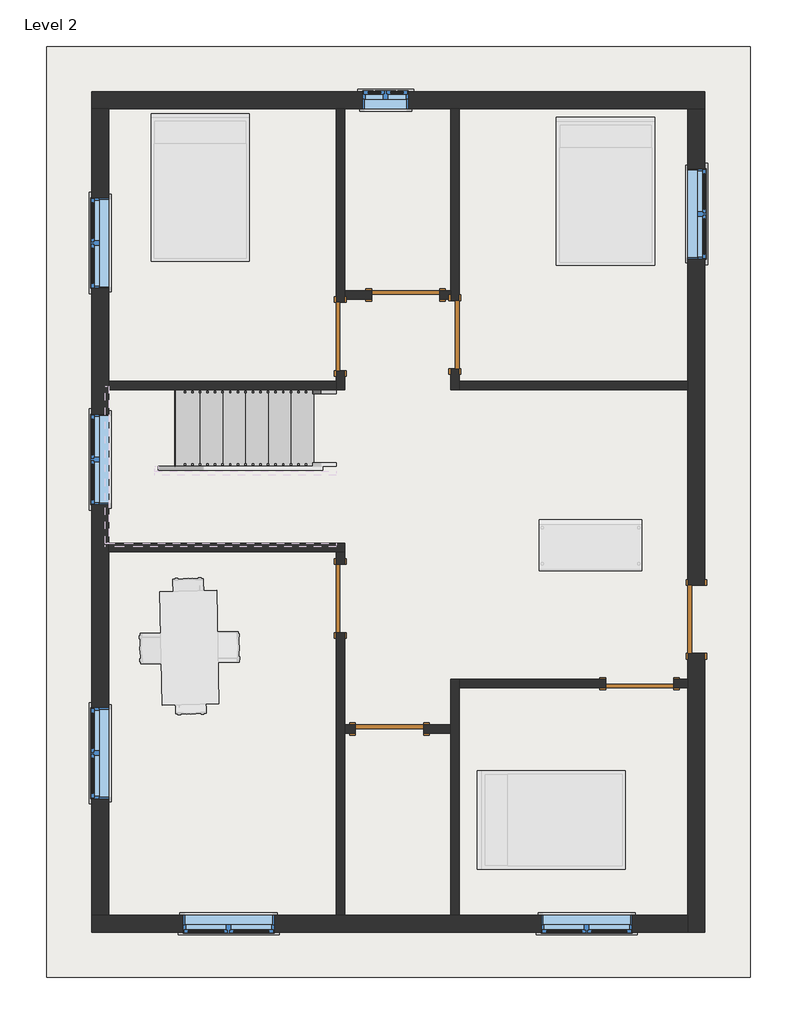
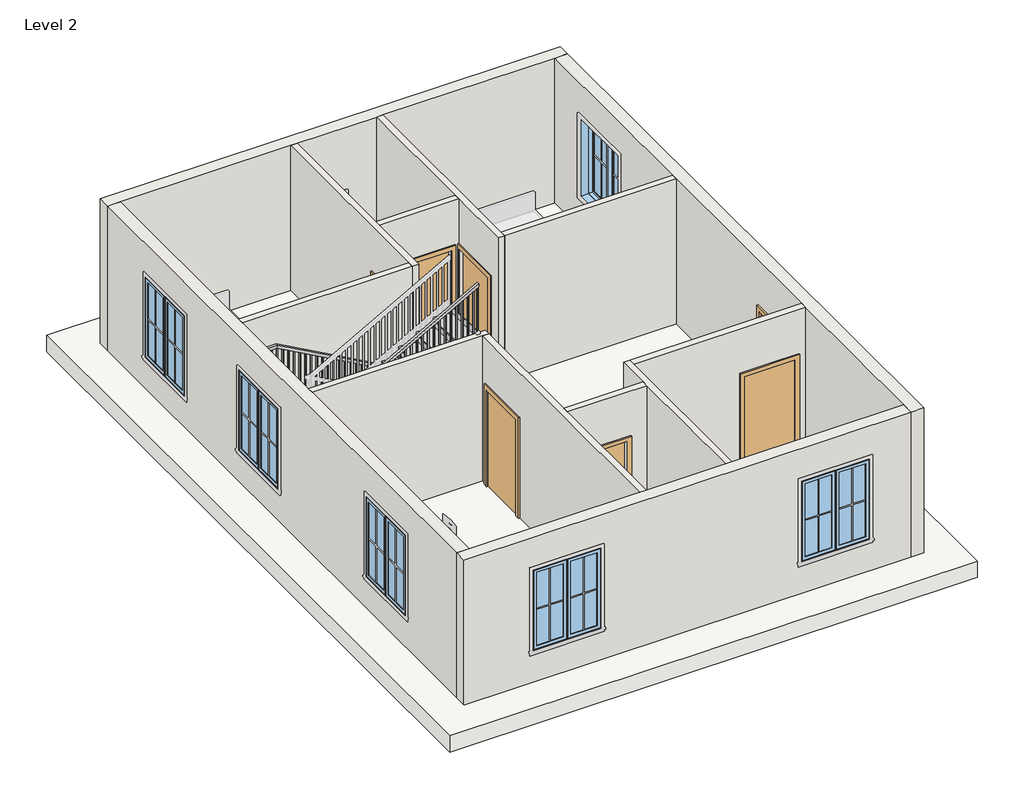
# One storey, part 1 of 2: 14 walls, 7 doors, 7 windows, 1 railing, 1 roof, 1 stair flight.
"""IFC4 building model written with IfcOpenShell, lengths in millimetres."""

from ifc_helpers import new_model, si_unit, frame, origin, place, context, project, spatial, polyline, outline, extrude, faceted_brep, transform, mapped, element, save
from components import door_e5f9f3c4, door_305aa2a5, door_a90ba1ad, stair_flight_289fc41f, window_c417fced, window_8377141f

model = new_model("IFC4")

# Units and contexts
model_context = context("Model", 3, world=origin())
ifc_project = project(units=[si_unit("LENGTHUNIT", "METRE", prefix="MILLI")], contexts=[model_context])

# Site, building, storey
site = spatial("IfcSite", under=ifc_project)
building = spatial("IfcBuilding", under=site)
storey = spatial("IfcBuildingStorey", under=building, Name="Level 2", Elevation=3048.0)

# Doors
placement = place(None, origin())
door_shape = door_e5f9f3c4(model_context)
element("IfcDoor", 1, ObjectType="Single-Flush : 36\" x 84\"", at=placement, inside=storey, context=model_context, shape_type="MappedRepresentation", body=[
    mapped(door_shape, transform((5226.05, 11245.85, 3048.0), x_axis=(1.0, 0.0, 0.0), y_axis=(0.0, 1.0, 0.0), z_axis=(0.0, 0.0, 1.0))),
])
element("IfcDoor", 2, ObjectType="Single-Flush : 36\" x 84\"", at=placement, inside=storey, context=model_context, shape_type="MappedRepresentation", body=[
    mapped(door_shape, transform((5886.45, 10712.45, 3048.0), x_axis=(0.0, -1.0, 0.0), y_axis=(1.0, 0.0, 0.0), z_axis=(0.0, 0.0, 1.0))),
])
door_2_shape = door_305aa2a5(model_context)
element("IfcDoor", 3, ObjectType="Single-Flush : 36\" x 84\"", at=placement, inside=storey, context=model_context, shape_type="MappedRepresentation", body=[
    mapped(door_2_shape, transform((4349.75, 10687.05, 3048.0), x_axis=(0.0, -1.0, 0.0), y_axis=(1.0, 0.0, 0.0), z_axis=(0.0, 0.0, 1.0))),
])
element("IfcDoor", 4, ObjectType="Single-Flush : 36\" x 84\"", at=placement, inside=storey, context=model_context, shape_type="MappedRepresentation", body=[
    mapped(door_2_shape, transform((8369.3, 6026.15, 3048.0), x_axis=(1.0, 0.0, 0.0), y_axis=(0.0, 1.0, 0.0), z_axis=(0.0, 0.0, 1.0))),
])
element("IfcDoor", 5, ObjectType="Single-Flush : 36\" x 84\"", at=placement, inside=storey, context=model_context, shape_type="MappedRepresentation", body=[
    mapped(door_2_shape, transform((5010.15, 5416.55, 3048.0), x_axis=(-1.0, 0.0, 0.0), y_axis=(0.0, -1.0, 0.0), z_axis=(0.0, 0.0, 1.0))),
])
element("IfcDoor", 6, ObjectType="Single-Flush : 36\" x 84\"", at=placement, inside=storey, context=model_context, shape_type="MappedRepresentation", body=[
    mapped(door_2_shape, transform((4349.75, 7169.15, 3048.0), x_axis=(0.0, -1.0, 0.0), y_axis=(1.0, 0.0, 0.0), z_axis=(0.0, 0.0, 1.0))),
])
door_3_shape = door_a90ba1ad(model_context)
element("IfcDoor", 7, ObjectType="Single-Flush : 36\" x 84\"", at=placement, inside=storey, context=model_context, shape_type="MappedRepresentation", body=[
    mapped(door_3_shape, transform((9131.3, 6889.75, 3048.0), x_axis=(0.0, -1.0, 0.0), y_axis=(1.0, 0.0, 0.0), z_axis=(0.0, 0.0, 1.0))),
])

# Railing
element("IfcRailing", 8, ObjectType="Handrail - Rectangular", at=placement, inside=storey, context=model_context, shape_type="SolidModel", body=[
    faceted_brep([(4295.1355783, 9918.7, 4131.7333333), (4295.1355783, 9918.7, 4073.620221), (4295.1355783, 9969.5, 4073.620221), (4295.1355783, 9969.5, 4131.7333333), (1856.7355783, 9918.7, 5486.4), (1843.5719761, 9918.7, 5435.6), (1843.5719761, 9969.5, 5435.6), (1856.7355783, 9969.5, 5486.4), (1295.4, 9918.7, 5486.4), (1295.4, 9918.7, 5435.6), (1244.6, 9969.5, 5435.6), (1244.6, 9969.5, 5486.4), (1295.4, 7962.9, 5486.4), (1295.4, 7962.9, 5435.6), (1244.6, 7912.1, 5435.6), (1244.6, 7912.1, 5486.4), (1551.9355783, 7962.9, 5486.4), (1565.0991806, 7962.9, 5435.6), (1565.0991806, 7912.1, 5435.6), (1551.9355783, 7912.1, 5486.4), (4295.1355783, 7962.9, 7010.4), (4295.1355783, 7912.1, 7010.4), (4295.1355783, 7912.1, 6952.2868876), (4295.1355783, 7962.9, 6952.2868876)], [[[0, 1, 2, 3]], [[1, 0, 4, 5]], [[2, 1, 5, 6]], [[3, 2, 6, 7]], [[0, 3, 7, 4]], [[5, 4, 8, 9]], [[6, 5, 9, 10]], [[7, 6, 10, 11]], [[4, 7, 11, 8]], [[9, 8, 12, 13]], [[10, 9, 13, 14]], [[11, 10, 14, 15]], [[8, 11, 15, 12]], [[13, 12, 16, 17]], [[14, 13, 17, 18]], [[15, 14, 18, 19]], [[12, 15, 19, 16]], [[20, 21, 22, 23]], [[17, 16, 20, 23]], [[18, 17, 23, 22]], [[19, 18, 22, 21]], [[16, 19, 21, 20]]]),
    extrude(outline(polyline([(6913.8365664, 4225.925), (6903.253233, 4206.875), (5926.6666667, 4206.875), (5926.6666667, 4225.925), (6913.8365664, 4225.925)])), frame((0.0, 7927.975, 0.0), z_axis=(0.0, 1.0, 0.0), x_axis=(0.0, 0.0, 1.0)), (0.0, 0.0, 1.0), 19.05),
    extrude(outline(polyline([(6857.3921219, 4124.325), (6846.8087886, 4105.275), (5926.6666667, 4105.275), (5926.6666667, 4124.325), (6857.3921219, 4124.325)])), frame((0.0, 7927.975, 0.0), z_axis=(0.0, 1.0, 0.0), x_axis=(0.0, 0.0, 1.0)), (0.0, 0.0, 1.0), 19.05),
    extrude(outline(polyline([(6800.9476775, 4022.725), (6790.3643441, 4003.675), (5926.6666667, 4003.675), (5926.6666667, 4022.725), (6800.9476775, 4022.725)])), frame((0.0, 7927.975, 0.0), z_axis=(0.0, 1.0, 0.0), x_axis=(0.0, 0.0, 1.0)), (0.0, 0.0, 1.0), 19.05),
    extrude(outline(polyline([(6744.503233, 3921.125), (6733.9198997, 3902.075), (5757.3333333, 3902.075), (5757.3333333, 3921.125), (6744.503233, 3921.125)])), frame((0.0, 7927.975, 0.0), z_axis=(0.0, 1.0, 0.0), x_axis=(0.0, 0.0, 1.0)), (0.0, 0.0, 1.0), 19.05),
    extrude(outline(polyline([(6688.0587886, 3819.525), (6677.4754552, 3800.475), (5757.3333333, 3800.475), (5757.3333333, 3819.525), (6688.0587886, 3819.525)])), frame((0.0, 7927.975, 0.0), z_axis=(0.0, 1.0, 0.0), x_axis=(0.0, 0.0, 1.0)), (0.0, 0.0, 1.0), 19.05),
    extrude(outline(polyline([(6631.6143441, 3717.925), (6621.0310108, 3698.875), (5757.3333333, 3698.875), (5757.3333333, 3717.925), (6631.6143441, 3717.925)])), frame((0.0, 7927.975, 0.0), z_axis=(0.0, 1.0, 0.0), x_axis=(0.0, 0.0, 1.0)), (0.0, 0.0, 1.0), 19.05),
    extrude(outline(polyline([(6575.1698997, 3616.325), (6564.5865664, 3597.275), (5588.0, 3597.275), (5588.0, 3616.325), (6575.1698997, 3616.325)])), frame((0.0, 7927.975, 0.0), z_axis=(0.0, 1.0, 0.0), x_axis=(0.0, 0.0, 1.0)), (0.0, 0.0, 1.0), 19.05),
    extrude(outline(polyline([(6518.7254552, 3514.725), (6508.1421219, 3495.675), (5588.0, 3495.675), (5588.0, 3514.725), (6518.7254552, 3514.725)])), frame((0.0, 7927.975, 0.0), z_axis=(0.0, 1.0, 0.0), x_axis=(0.0, 0.0, 1.0)), (0.0, 0.0, 1.0), 19.05),
    extrude(outline(polyline([(6462.2810108, 3413.125), (6451.6976775, 3394.075), (5588.0, 3394.075), (5588.0, 3413.125), (6462.2810108, 3413.125)])), frame((0.0, 7927.975, 0.0), z_axis=(0.0, 1.0, 0.0), x_axis=(0.0, 0.0, 1.0)), (0.0, 0.0, 1.0), 19.05),
    extrude(outline(polyline([(6405.8365664, 3311.525), (6395.253233, 3292.475), (5418.6666667, 3292.475), (5418.6666667, 3311.525), (6405.8365664, 3311.525)])), frame((0.0, 7927.975, 0.0), z_axis=(0.0, 1.0, 0.0), x_axis=(0.0, 0.0, 1.0)), (0.0, 0.0, 1.0), 19.05),
    extrude(outline(polyline([(6349.3921219, 3209.925), (6338.8087886, 3190.875), (5418.6666667, 3190.875), (5418.6666667, 3209.925), (6349.3921219, 3209.925)])), frame((0.0, 7927.975, 0.0), z_axis=(0.0, 1.0, 0.0), x_axis=(0.0, 0.0, 1.0)), (0.0, 0.0, 1.0), 19.05),
    extrude(outline(polyline([(6292.9476775, 3108.325), (6282.3643441, 3089.275), (5418.6666667, 3089.275), (5418.6666667, 3108.325), (6292.9476775, 3108.325)])), frame((0.0, 7927.975, 0.0), z_axis=(0.0, 1.0, 0.0), x_axis=(0.0, 0.0, 1.0)), (0.0, 0.0, 1.0), 19.05),
    extrude(outline(polyline([(6236.503233, 3006.725), (6225.9198997, 2987.675), (5249.3333333, 2987.675), (5249.3333333, 3006.725), (6236.503233, 3006.725)])), frame((0.0, 7927.975, 0.0), z_axis=(0.0, 1.0, 0.0), x_axis=(0.0, 0.0, 1.0)), (0.0, 0.0, 1.0), 19.05),
    extrude(outline(polyline([(6180.0587886, 2905.125), (6169.4754552, 2886.075), (5249.3333333, 2886.075), (5249.3333333, 2905.125), (6180.0587886, 2905.125)])), frame((0.0, 7927.975, 0.0), z_axis=(0.0, 1.0, 0.0), x_axis=(0.0, 0.0, 1.0)), (0.0, 0.0, 1.0), 19.05),
    extrude(outline(polyline([(6123.6143441, 2803.525), (6113.0310108, 2784.475), (5249.3333333, 2784.475), (5249.3333333, 2803.525), (6123.6143441, 2803.525)])), frame((0.0, 7927.975, 0.0), z_axis=(0.0, 1.0, 0.0), x_axis=(0.0, 0.0, 1.0)), (0.0, 0.0, 1.0), 19.05),
    extrude(outline(polyline([(6067.1698997, 2701.925), (6056.5865664, 2682.875), (5080.0, 2682.875), (5080.0, 2701.925), (6067.1698997, 2701.925)])), frame((0.0, 7927.975, 0.0), z_axis=(0.0, 1.0, 0.0), x_axis=(0.0, 0.0, 1.0)), (0.0, 0.0, 1.0), 19.05),
    extrude(outline(polyline([(6010.7254552, 2600.325), (6000.1421219, 2581.275), (5080.0, 2581.275), (5080.0, 2600.325), (6010.7254552, 2600.325)])), frame((0.0, 7927.975, 0.0), z_axis=(0.0, 1.0, 0.0), x_axis=(0.0, 0.0, 1.0)), (0.0, 0.0, 1.0), 19.05),
    extrude(outline(polyline([(5954.2810108, 2498.725), (5943.6976775, 2479.675), (5080.0, 2479.675), (5080.0, 2498.725), (5954.2810108, 2498.725)])), frame((0.0, 7927.975, 0.0), z_axis=(0.0, 1.0, 0.0), x_axis=(0.0, 0.0, 1.0)), (0.0, 0.0, 1.0), 19.05),
    extrude(outline(polyline([(5897.8365664, 2397.125), (5887.253233, 2378.075), (4910.6666667, 2378.075), (4910.6666667, 2397.125), (5897.8365664, 2397.125)])), frame((0.0, 7927.975, 0.0), z_axis=(0.0, 1.0, 0.0), x_axis=(0.0, 0.0, 1.0)), (0.0, 0.0, 1.0), 19.05),
    extrude(outline(polyline([(5841.3921219, 2295.525), (5830.8087886, 2276.475), (4910.6666667, 2276.475), (4910.6666667, 2295.525), (5841.3921219, 2295.525)])), frame((0.0, 7927.975, 0.0), z_axis=(0.0, 1.0, 0.0), x_axis=(0.0, 0.0, 1.0)), (0.0, 0.0, 1.0), 19.05),
    extrude(outline(polyline([(5784.9476775, 2193.925), (5774.3643441, 2174.875), (4910.6666667, 2174.875), (4910.6666667, 2193.925), (5784.9476775, 2193.925)])), frame((0.0, 7927.975, 0.0), z_axis=(0.0, 1.0, 0.0), x_axis=(0.0, 0.0, 1.0)), (0.0, 0.0, 1.0), 19.05),
    extrude(outline(polyline([(5728.503233, 2092.325), (5717.9198997, 2073.275), (4741.3333333, 2073.275), (4741.3333333, 2092.325), (5728.503233, 2092.325)])), frame((0.0, 7927.975, 0.0), z_axis=(0.0, 1.0, 0.0), x_axis=(0.0, 0.0, 1.0)), (0.0, 0.0, 1.0), 19.05),
    extrude(outline(polyline([(5672.0587886, 1990.725), (5661.4754552, 1971.675), (4741.3333333, 1971.675), (4741.3333333, 1990.725), (5672.0587886, 1990.725)])), frame((0.0, 7927.975, 0.0), z_axis=(0.0, 1.0, 0.0), x_axis=(0.0, 0.0, 1.0)), (0.0, 0.0, 1.0), 19.05),
    extrude(outline(polyline([(5615.6143441, 1889.125), (5605.0310108, 1870.075), (4741.3333333, 1870.075), (4741.3333333, 1889.125), (5615.6143441, 1889.125)])), frame((0.0, 7927.975, 0.0), z_axis=(0.0, 1.0, 0.0), x_axis=(0.0, 0.0, 1.0)), (0.0, 0.0, 1.0), 19.05),
    extrude(outline(polyline([(5559.1698997, 1787.525), (5548.5865664, 1768.475), (4572.0, 1768.475), (4572.0, 1787.525), (5559.1698997, 1787.525)])), frame((0.0, 7927.975, 0.0), z_axis=(0.0, 1.0, 0.0), x_axis=(0.0, 0.0, 1.0)), (0.0, 0.0, 1.0), 19.05),
    extrude(outline(polyline([(5502.7254552, 1685.925), (5492.1421219, 1666.875), (4572.0, 1666.875), (4572.0, 1685.925), (5502.7254552, 1685.925)])), frame((0.0, 7927.975, 0.0), z_axis=(0.0, 1.0, 0.0), x_axis=(0.0, 0.0, 1.0)), (0.0, 0.0, 1.0), 19.05),
    extrude(outline(polyline([(5446.2810108, 1584.325), (5435.6976775, 1565.275), (4572.0, 1565.275), (4572.0, 1584.325), (5446.2810108, 1584.325)])), frame((0.0, 7927.975, 0.0), z_axis=(0.0, 1.0, 0.0), x_axis=(0.0, 0.0, 1.0)), (0.0, 0.0, 1.0), 19.05),
    extrude(outline(polyline([(1463.675, 7927.975), (1463.675, 7947.025), (1482.725, 7947.025), (1482.725, 7927.975), (1463.675, 7927.975)])), frame((0.0, 0.0, 4572.0), z_axis=(0.0, 0.0, 1.0), x_axis=(1.0, 0.0, 0.0)), (0.0, 0.0, 1.0), 863.6),
    extrude(outline(polyline([(1362.075, 7927.975), (1362.075, 7947.025), (1381.125, 7947.025), (1381.125, 7927.975), (1362.075, 7927.975)])), frame((0.0, 0.0, 4572.0), z_axis=(0.0, 0.0, 1.0), x_axis=(1.0, 0.0, 0.0)), (0.0, 0.0, 1.0), 863.6),
    extrude(outline(polyline([(1260.475, 8023.225), (1279.525, 8023.225), (1279.525, 8004.175), (1260.475, 8004.175), (1260.475, 8023.225)])), frame((0.0, 0.0, 4572.0), z_axis=(0.0, 0.0, 1.0), x_axis=(1.0, 0.0, 0.0)), (0.0, 0.0, 1.0), 863.6),
    extrude(outline(polyline([(1260.475, 8124.825), (1279.525, 8124.825), (1279.525, 8105.775), (1260.475, 8105.775), (1260.475, 8124.825)])), frame((0.0, 0.0, 4572.0), z_axis=(0.0, 0.0, 1.0), x_axis=(1.0, 0.0, 0.0)), (0.0, 0.0, 1.0), 863.6),
    extrude(outline(polyline([(1260.475, 8226.425), (1279.525, 8226.425), (1279.525, 8207.375), (1260.475, 8207.375), (1260.475, 8226.425)])), frame((0.0, 0.0, 4572.0), z_axis=(0.0, 0.0, 1.0), x_axis=(1.0, 0.0, 0.0)), (0.0, 0.0, 1.0), 863.6),
    extrude(outline(polyline([(1260.475, 8328.025), (1279.525, 8328.025), (1279.525, 8308.975), (1260.475, 8308.975), (1260.475, 8328.025)])), frame((0.0, 0.0, 4572.0), z_axis=(0.0, 0.0, 1.0), x_axis=(1.0, 0.0, 0.0)), (0.0, 0.0, 1.0), 863.6),
    extrude(outline(polyline([(1260.475, 8429.625), (1279.525, 8429.625), (1279.525, 8410.575), (1260.475, 8410.575), (1260.475, 8429.625)])), frame((0.0, 0.0, 4572.0), z_axis=(0.0, 0.0, 1.0), x_axis=(1.0, 0.0, 0.0)), (0.0, 0.0, 1.0), 863.6),
    extrude(outline(polyline([(1260.475, 8531.225), (1279.525, 8531.225), (1279.525, 8512.175), (1260.475, 8512.175), (1260.475, 8531.225)])), frame((0.0, 0.0, 4572.0), z_axis=(0.0, 0.0, 1.0), x_axis=(1.0, 0.0, 0.0)), (0.0, 0.0, 1.0), 863.6),
    extrude(outline(polyline([(1260.475, 8632.825), (1279.525, 8632.825), (1279.525, 8613.775), (1260.475, 8613.775), (1260.475, 8632.825)])), frame((0.0, 0.0, 4572.0), z_axis=(0.0, 0.0, 1.0), x_axis=(1.0, 0.0, 0.0)), (0.0, 0.0, 1.0), 863.6),
    extrude(outline(polyline([(1260.475, 8734.425), (1279.525, 8734.425), (1279.525, 8715.375), (1260.475, 8715.375), (1260.475, 8734.425)])), frame((0.0, 0.0, 4572.0), z_axis=(0.0, 0.0, 1.0), x_axis=(1.0, 0.0, 0.0)), (0.0, 0.0, 1.0), 863.6),
    extrude(outline(polyline([(1260.475, 8836.025), (1279.525, 8836.025), (1279.525, 8816.975), (1260.475, 8816.975), (1260.475, 8836.025)])), frame((0.0, 0.0, 4572.0), z_axis=(0.0, 0.0, 1.0), x_axis=(1.0, 0.0, 0.0)), (0.0, 0.0, 1.0), 863.6),
    extrude(outline(polyline([(1260.475, 8937.625), (1279.525, 8937.625), (1279.525, 8918.575), (1260.475, 8918.575), (1260.475, 8937.625)])), frame((0.0, 0.0, 4572.0), z_axis=(0.0, 0.0, 1.0), x_axis=(1.0, 0.0, 0.0)), (0.0, 0.0, 1.0), 863.6),
    extrude(outline(polyline([(1260.475, 9039.225), (1279.525, 9039.225), (1279.525, 9020.175), (1260.475, 9020.175), (1260.475, 9039.225)])), frame((0.0, 0.0, 4572.0), z_axis=(0.0, 0.0, 1.0), x_axis=(1.0, 0.0, 0.0)), (0.0, 0.0, 1.0), 863.6),
    extrude(outline(polyline([(1260.475, 9140.825), (1279.525, 9140.825), (1279.525, 9121.775), (1260.475, 9121.775), (1260.475, 9140.825)])), frame((0.0, 0.0, 4572.0), z_axis=(0.0, 0.0, 1.0), x_axis=(1.0, 0.0, 0.0)), (0.0, 0.0, 1.0), 863.6),
    extrude(outline(polyline([(1260.475, 9242.425), (1279.525, 9242.425), (1279.525, 9223.375), (1260.475, 9223.375), (1260.475, 9242.425)])), frame((0.0, 0.0, 4572.0), z_axis=(0.0, 0.0, 1.0), x_axis=(1.0, 0.0, 0.0)), (0.0, 0.0, 1.0), 863.6),
    extrude(outline(polyline([(1260.475, 9344.025), (1279.525, 9344.025), (1279.525, 9324.975), (1260.475, 9324.975), (1260.475, 9344.025)])), frame((0.0, 0.0, 4572.0), z_axis=(0.0, 0.0, 1.0), x_axis=(1.0, 0.0, 0.0)), (0.0, 0.0, 1.0), 863.6),
    extrude(outline(polyline([(1260.475, 9445.625), (1279.525, 9445.625), (1279.525, 9426.575), (1260.475, 9426.575), (1260.475, 9445.625)])), frame((0.0, 0.0, 4572.0), z_axis=(0.0, 0.0, 1.0), x_axis=(1.0, 0.0, 0.0)), (0.0, 0.0, 1.0), 863.6),
    extrude(outline(polyline([(1260.475, 9547.225), (1279.525, 9547.225), (1279.525, 9528.175), (1260.475, 9528.175), (1260.475, 9547.225)])), frame((0.0, 0.0, 4572.0), z_axis=(0.0, 0.0, 1.0), x_axis=(1.0, 0.0, 0.0)), (0.0, 0.0, 1.0), 863.6),
    extrude(outline(polyline([(1260.475, 9648.825), (1279.525, 9648.825), (1279.525, 9629.775), (1260.475, 9629.775), (1260.475, 9648.825)])), frame((0.0, 0.0, 4572.0), z_axis=(0.0, 0.0, 1.0), x_axis=(1.0, 0.0, 0.0)), (0.0, 0.0, 1.0), 863.6),
    extrude(outline(polyline([(1260.475, 9750.425), (1279.525, 9750.425), (1279.525, 9731.375), (1260.475, 9731.375), (1260.475, 9750.425)])), frame((0.0, 0.0, 4572.0), z_axis=(0.0, 0.0, 1.0), x_axis=(1.0, 0.0, 0.0)), (0.0, 0.0, 1.0), 863.6),
    extrude(outline(polyline([(1260.475, 9852.025), (1279.525, 9852.025), (1279.525, 9832.975), (1260.475, 9832.975), (1260.475, 9852.025)])), frame((0.0, 0.0, 4572.0), z_axis=(0.0, 0.0, 1.0), x_axis=(1.0, 0.0, 0.0)), (0.0, 0.0, 1.0), 863.6),
    extrude(outline(polyline([(1358.2605783, 9953.625), (1358.2605783, 9934.575), (1339.2105783, 9934.575), (1339.2105783, 9953.625), (1358.2605783, 9953.625)])), frame((0.0, 0.0, 4572.0), z_axis=(0.0, 0.0, 1.0), x_axis=(1.0, 0.0, 0.0)), (0.0, 0.0, 1.0), 863.6),
    extrude(outline(polyline([(1459.8605783, 9953.625), (1459.8605783, 9934.575), (1440.8105783, 9934.575), (1440.8105783, 9953.625), (1459.8605783, 9953.625)])), frame((0.0, 0.0, 4572.0), z_axis=(0.0, 0.0, 1.0), x_axis=(1.0, 0.0, 0.0)), (0.0, 0.0, 1.0), 863.6),
    extrude(outline(polyline([(1561.4605783, 9953.625), (1561.4605783, 9934.575), (1542.4105783, 9934.575), (1542.4105783, 9953.625), (1561.4605783, 9953.625)])), frame((0.0, 0.0, 4572.0), z_axis=(0.0, 0.0, 1.0), x_axis=(1.0, 0.0, 0.0)), (0.0, 0.0, 1.0), 863.6),
    extrude(outline(polyline([(1663.0605783, 9953.625), (1663.0605783, 9934.575), (1644.0105783, 9934.575), (1644.0105783, 9953.625), (1663.0605783, 9953.625)])), frame((0.0, 0.0, 4572.0), z_axis=(0.0, 0.0, 1.0), x_axis=(1.0, 0.0, 0.0)), (0.0, 0.0, 1.0), 863.6),
    extrude(outline(polyline([(1764.6605783, 9953.625), (1764.6605783, 9934.575), (1745.6105783, 9934.575), (1745.6105783, 9953.625), (1764.6605783, 9953.625)])), frame((0.0, 0.0, 4572.0), z_axis=(0.0, 0.0, 1.0), x_axis=(1.0, 0.0, 0.0)), (0.0, 0.0, 1.0), 863.6),
    extrude(outline(polyline([(5422.995221, 1866.2605783), (5433.5785543, 1847.2105783), (4572.0, 1847.2105783), (4572.0, 1866.2605783), (5422.995221, 1866.2605783)])), frame((0.0, 9934.575, 0.0), z_axis=(0.0, 1.0, 0.0), x_axis=(0.0, 0.0, 1.0)), (0.0, 0.0, 1.0), 19.05),
    extrude(outline(polyline([(5366.5507765, 1967.8605783), (5377.1341099, 1948.8105783), (4402.6666667, 1948.8105783), (4402.6666667, 1967.8605783), (5366.5507765, 1967.8605783)])), frame((0.0, 9934.575, 0.0), z_axis=(0.0, 1.0, 0.0), x_axis=(0.0, 0.0, 1.0)), (0.0, 0.0, 1.0), 19.05),
    extrude(outline(polyline([(5310.1063321, 2069.4605783), (5320.6896654, 2050.4105783), (4402.6666667, 2050.4105783), (4402.6666667, 2069.4605783), (5310.1063321, 2069.4605783)])), frame((0.0, 9934.575, 0.0), z_axis=(0.0, 1.0, 0.0), x_axis=(0.0, 0.0, 1.0)), (0.0, 0.0, 1.0), 19.05),
    extrude(outline(polyline([(5253.6618876, 2171.0605783), (5264.245221, 2152.0105783), (4402.6666667, 2152.0105783), (4402.6666667, 2171.0605783), (5253.6618876, 2171.0605783)])), frame((0.0, 9934.575, 0.0), z_axis=(0.0, 1.0, 0.0), x_axis=(0.0, 0.0, 1.0)), (0.0, 0.0, 1.0), 19.05),
    extrude(outline(polyline([(5197.2174432, 2272.6605783), (5207.8007765, 2253.6105783), (4233.3333333, 2253.6105783), (4233.3333333, 2272.6605783), (5197.2174432, 2272.6605783)])), frame((0.0, 9934.575, 0.0), z_axis=(0.0, 1.0, 0.0), x_axis=(0.0, 0.0, 1.0)), (0.0, 0.0, 1.0), 19.05),
    extrude(outline(polyline([(5140.7729988, 2374.2605783), (5151.3563321, 2355.2105783), (4233.3333333, 2355.2105783), (4233.3333333, 2374.2605783), (5140.7729988, 2374.2605783)])), frame((0.0, 9934.575, 0.0), z_axis=(0.0, 1.0, 0.0), x_axis=(0.0, 0.0, 1.0)), (0.0, 0.0, 1.0), 19.05),
    extrude(outline(polyline([(5084.3285543, 2475.8605783), (5094.9118876, 2456.8105783), (4233.3333333, 2456.8105783), (4233.3333333, 2475.8605783), (5084.3285543, 2475.8605783)])), frame((0.0, 9934.575, 0.0), z_axis=(0.0, 1.0, 0.0), x_axis=(0.0, 0.0, 1.0)), (0.0, 0.0, 1.0), 19.05),
    extrude(outline(polyline([(5027.8841099, 2577.4605783), (5038.4674432, 2558.4105783), (4064.0, 2558.4105783), (4064.0, 2577.4605783), (5027.8841099, 2577.4605783)])), frame((0.0, 9934.575, 0.0), z_axis=(0.0, 1.0, 0.0), x_axis=(0.0, 0.0, 1.0)), (0.0, 0.0, 1.0), 19.05),
    extrude(outline(polyline([(4971.4396654, 2679.0605783), (4982.0229988, 2660.0105783), (4064.0, 2660.0105783), (4064.0, 2679.0605783), (4971.4396654, 2679.0605783)])), frame((0.0, 9934.575, 0.0), z_axis=(0.0, 1.0, 0.0), x_axis=(0.0, 0.0, 1.0)), (0.0, 0.0, 1.0), 19.05),
    extrude(outline(polyline([(4914.995221, 2780.6605783), (4925.5785543, 2761.6105783), (4064.0, 2761.6105783), (4064.0, 2780.6605783), (4914.995221, 2780.6605783)])), frame((0.0, 9934.575, 0.0), z_axis=(0.0, 1.0, 0.0), x_axis=(0.0, 0.0, 1.0)), (0.0, 0.0, 1.0), 19.05),
    extrude(outline(polyline([(4858.5507765, 2882.2605783), (4869.1341099, 2863.2105783), (3894.6666667, 2863.2105783), (3894.6666667, 2882.2605783), (4858.5507765, 2882.2605783)])), frame((0.0, 9934.575, 0.0), z_axis=(0.0, 1.0, 0.0), x_axis=(0.0, 0.0, 1.0)), (0.0, 0.0, 1.0), 19.05),
    extrude(outline(polyline([(4802.1063321, 2983.8605783), (4812.6896654, 2964.8105783), (3894.6666667, 2964.8105783), (3894.6666667, 2983.8605783), (4802.1063321, 2983.8605783)])), frame((0.0, 9934.575, 0.0), z_axis=(0.0, 1.0, 0.0), x_axis=(0.0, 0.0, 1.0)), (0.0, 0.0, 1.0), 19.05),
    extrude(outline(polyline([(4745.6618876, 3085.4605783), (4756.245221, 3066.4105783), (3894.6666667, 3066.4105783), (3894.6666667, 3085.4605783), (4745.6618876, 3085.4605783)])), frame((0.0, 9934.575, 0.0), z_axis=(0.0, 1.0, 0.0), x_axis=(0.0, 0.0, 1.0)), (0.0, 0.0, 1.0), 19.05),
    extrude(outline(polyline([(4689.2174432, 3187.0605783), (4699.8007765, 3168.0105783), (3725.3333333, 3168.0105783), (3725.3333333, 3187.0605783), (4689.2174432, 3187.0605783)])), frame((0.0, 9934.575, 0.0), z_axis=(0.0, 1.0, 0.0), x_axis=(0.0, 0.0, 1.0)), (0.0, 0.0, 1.0), 19.05),
    extrude(outline(polyline([(4632.7729988, 3288.6605783), (4643.3563321, 3269.6105783), (3725.3333333, 3269.6105783), (3725.3333333, 3288.6605783), (4632.7729988, 3288.6605783)])), frame((0.0, 9934.575, 0.0), z_axis=(0.0, 1.0, 0.0), x_axis=(0.0, 0.0, 1.0)), (0.0, 0.0, 1.0), 19.05),
    extrude(outline(polyline([(4576.3285543, 3390.2605783), (4586.9118876, 3371.2105783), (3725.3333333, 3371.2105783), (3725.3333333, 3390.2605783), (4576.3285543, 3390.2605783)])), frame((0.0, 9934.575, 0.0), z_axis=(0.0, 1.0, 0.0), x_axis=(0.0, 0.0, 1.0)), (0.0, 0.0, 1.0), 19.05),
    extrude(outline(polyline([(4519.8841099, 3491.8605783), (4530.4674432, 3472.8105783), (3556.0, 3472.8105783), (3556.0, 3491.8605783), (4519.8841099, 3491.8605783)])), frame((0.0, 9934.575, 0.0), z_axis=(0.0, 1.0, 0.0), x_axis=(0.0, 0.0, 1.0)), (0.0, 0.0, 1.0), 19.05),
    extrude(outline(polyline([(4463.4396654, 3593.4605783), (4474.0229988, 3574.4105783), (3556.0, 3574.4105783), (3556.0, 3593.4605783), (4463.4396654, 3593.4605783)])), frame((0.0, 9934.575, 0.0), z_axis=(0.0, 1.0, 0.0), x_axis=(0.0, 0.0, 1.0)), (0.0, 0.0, 1.0), 19.05),
    extrude(outline(polyline([(4406.995221, 3695.0605783), (4417.5785543, 3676.0105783), (3556.0, 3676.0105783), (3556.0, 3695.0605783), (4406.995221, 3695.0605783)])), frame((0.0, 9934.575, 0.0), z_axis=(0.0, 1.0, 0.0), x_axis=(0.0, 0.0, 1.0)), (0.0, 0.0, 1.0), 19.05),
    extrude(outline(polyline([(4350.5507765, 3796.6605783), (4361.1341099, 3777.6105783), (3386.6666667, 3777.6105783), (3386.6666667, 3796.6605783), (4350.5507765, 3796.6605783)])), frame((0.0, 9934.575, 0.0), z_axis=(0.0, 1.0, 0.0), x_axis=(0.0, 0.0, 1.0)), (0.0, 0.0, 1.0), 19.05),
    extrude(outline(polyline([(4294.1063321, 3898.2605783), (4304.6896654, 3879.2105783), (3386.6666667, 3879.2105783), (3386.6666667, 3898.2605783), (4294.1063321, 3898.2605783)])), frame((0.0, 9934.575, 0.0), z_axis=(0.0, 1.0, 0.0), x_axis=(0.0, 0.0, 1.0)), (0.0, 0.0, 1.0), 19.05),
    extrude(outline(polyline([(4237.6618876, 3999.8605783), (4248.245221, 3980.8105783), (3386.6666667, 3980.8105783), (3386.6666667, 3999.8605783), (4237.6618876, 3999.8605783)])), frame((0.0, 9934.575, 0.0), z_axis=(0.0, 1.0, 0.0), x_axis=(0.0, 0.0, 1.0)), (0.0, 0.0, 1.0), 19.05),
    extrude(outline(polyline([(4181.2174432, 4101.4605783), (4191.8007765, 4082.4105783), (3217.3333333, 4082.4105783), (3217.3333333, 4101.4605783), (4181.2174432, 4101.4605783)])), frame((0.0, 9934.575, 0.0), z_axis=(0.0, 1.0, 0.0), x_axis=(0.0, 0.0, 1.0)), (0.0, 0.0, 1.0), 19.05),
    extrude(outline(polyline([(4124.7729988, 4203.0605783), (4135.3563321, 4184.0105783), (3217.3333333, 4184.0105783), (3217.3333333, 4203.0605783), (4124.7729988, 4203.0605783)])), frame((0.0, 9934.575, 0.0), z_axis=(0.0, 1.0, 0.0), x_axis=(0.0, 0.0, 1.0)), (0.0, 0.0, 1.0), 19.05),
    extrude(outline(polyline([(1260.475, 7947.025), (1279.525, 7947.025), (1279.525, 7927.975), (1260.475, 7927.975), (1260.475, 7947.025)])), frame((0.0, 0.0, 4572.0), z_axis=(0.0, 0.0, 1.0), x_axis=(1.0, 0.0, 0.0)), (0.0, 0.0, 1.0), 863.6),
    extrude(outline(polyline([(1279.525, 9953.625), (1279.525, 9934.575), (1260.475, 9934.575), (1260.475, 9953.625), (1279.525, 9953.625)])), frame((0.0, 0.0, 4572.0), z_axis=(0.0, 0.0, 1.0), x_axis=(1.0, 0.0, 0.0)), (0.0, 0.0, 1.0), 863.6),
    extrude(outline(polyline([(6952.2868876, 4295.1355783), (6941.7035543, 4276.0855783), (5926.6666667, 4276.0855783), (5926.6666667, 4295.1355783), (6952.2868876, 4295.1355783)])), frame((0.0, 7927.975, 0.0), z_axis=(0.0, 1.0, 0.0), x_axis=(0.0, 0.0, 1.0)), (0.0, 0.0, 1.0), 19.05),
    extrude(outline(polyline([(4073.620221, 4295.1355783), (4084.2035543, 4276.0855783), (3217.3333333, 4276.0855783), (3217.3333333, 4295.1355783), (4073.620221, 4295.1355783)])), frame((0.0, 9934.575, 0.0), z_axis=(0.0, 1.0, 0.0), x_axis=(0.0, 0.0, 1.0)), (0.0, 0.0, 1.0), 19.05),
])

# Roof
element("IfcRoof", 9, ObjectType="Generic - 12\"", at=placement, inside=storey, context=model_context, shape_type="SweptSolid", body=[
    extrude(outline(polyline([(406.4, 14579.6), (9855.2, 14579.6), (9855.2, 2082.8), (406.4, 2082.8), (406.4, 14579.6)])), frame((0.0, 0.0, 3048.0), z_axis=(0.0, 0.0, 1.0), x_axis=(1.0, 0.0, 0.0)), (0.0, 0.0, 1.0), 304.8),
])

# Stair flight
stair_flight_shape = stair_flight_289fc41f(model_context)
element("IfcStairFlight", 10, ObjectType="2\" Tread 1\" Nosing 1/4\" Riser", at=placement, inside=storey, context=model_context, shape_type="MappedRepresentation", body=[
    mapped(stair_flight_shape, transform((0.0, 0.0, 0.0), x_axis=(1.0, 0.0, 0.0), y_axis=(0.0, 1.0, 0.0), z_axis=(0.0, 0.0, 1.0))),
])

# Walls
element("IfcWall", 11, ObjectType="Generic - 5\"", at=placement, inside=storey, context=model_context, shape_type="Brep", body=[
    faceted_brep([(4292.6, 10229.85, 5181.6), (4292.6, 10229.85, 3048.0), (4292.6, 10083.8, 3048.0), (4292.6, 9969.5, 3048.0), (4292.6, 9969.5, 6096.0), (4292.6, 10083.8, 6096.0), (4292.6, 13741.4, 6096.0), (4292.6, 13741.4, 3048.0), (4292.6, 11144.25, 3048.0), (4292.6, 11144.25, 5181.6), (4406.9, 9969.5, 3048.0), (4406.9, 10229.85, 3048.0), (4406.9, 10229.85, 5181.6), (4406.9, 11144.25, 5181.6), (4406.9, 11144.25, 3048.0), (4406.9, 11188.7, 3048.0), (4406.9, 11303.0, 3048.0), (4406.9, 13741.4, 3048.0), (4406.9, 13741.4, 6096.0), (4406.9, 11303.0, 6096.0), (4406.9, 11188.7, 6096.0), (4406.9, 9969.5, 6096.0)], [[[0, 1, 2, 3, 4, 5, 6, 7, 8, 9]], [[10, 11, 12, 13, 14, 15, 16, 17, 18, 19, 20, 21]], [[8, 7, 17, 16, 15, 14]], [[3, 2, 1, 11, 10]], [[6, 5, 4, 21, 20, 19, 18]], [[7, 6, 18, 17]], [[4, 3, 10, 21]], [[12, 11, 1, 0]], [[13, 12, 0, 9]], [[14, 13, 9, 8]]]),
])
element("IfcWall", 12, ObjectType="Generic - 5\"", at=placement, inside=storey, context=model_context, shape_type="SweptSolid", body=[
    extrude(outline(polyline([(1244.6, 10083.8), (4292.6, 10083.8), (4292.6, 9969.5), (1244.6, 9969.5), (1244.6, 10083.8)])), frame((0.0, 0.0, 3048.0), z_axis=(0.0, 0.0, 1.0), x_axis=(1.0, 0.0, 0.0)), (0.0, 0.0, 1.0), 3048.0),
])
element("IfcWall", 13, ObjectType="Generic - 5\"", at=placement, inside=storey, context=model_context, shape_type="SweptSolid", body=[
    extrude(outline(polyline([(5181.6, 5683.25), (3048.0, 5683.25), (3048.0, 5829.3), (6096.0, 5829.3), (6096.0, 4406.9), (3048.0, 4406.9), (3048.0, 4768.85), (5181.6, 4768.85), (5181.6, 5683.25)])), frame((0.0, 11188.7, 0.0), z_axis=(0.0, 1.0, 0.0), x_axis=(0.0, 0.0, 1.0)), (0.0, 0.0, 1.0), 114.3),
])
element("IfcWall", 14, ObjectType="Generic - 5\"", at=placement, inside=storey, context=model_context, shape_type="Brep", body=[
    faceted_brep([(5829.3, 10255.25, 5181.6), (5829.3, 10255.25, 3048.0), (5829.3, 9969.5, 3048.0), (5829.3, 9969.5, 6096.0), (5829.3, 11188.7, 6096.0), (5829.3, 11303.0, 6096.0), (5829.3, 13741.4, 6096.0), (5829.3, 13741.4, 3048.0), (5829.3, 11303.0, 3048.0), (5829.3, 11188.7, 3048.0), (5829.3, 11169.65, 3048.0), (5829.3, 11169.65, 5181.6), (5943.6, 9969.5, 3048.0), (5943.6, 10083.8, 3048.0), (5943.6, 10255.25, 3048.0), (5943.6, 10255.25, 5181.6), (5943.6, 11169.65, 5181.6), (5943.6, 11169.65, 3048.0), (5943.6, 13741.4, 3048.0), (5943.6, 13741.4, 6096.0), (5943.6, 10083.8, 6096.0), (5943.6, 9969.5, 6096.0)], [[[0, 1, 2, 3, 4, 5, 6, 7, 8, 9, 10, 11]], [[12, 13, 14, 15, 16, 17, 18, 19, 20, 21]], [[2, 1, 14, 13, 12]], [[10, 9, 8, 7, 18, 17]], [[6, 5, 4, 3, 21, 20, 19]], [[7, 6, 19, 18]], [[3, 2, 12, 21]], [[15, 14, 1, 0]], [[16, 15, 0, 11]], [[17, 16, 11, 10]]]),
])
element("IfcWall", 15, ObjectType="Generic - 5\"", at=placement, inside=storey, context=model_context, shape_type="SweptSolid", body=[
    extrude(outline(polyline([(9017.0, 9969.5), (5943.6, 9969.5), (5943.6, 10083.8), (9017.0, 10083.8), (9017.0, 9969.5)])), frame((0.0, 0.0, 3048.0), z_axis=(0.0, 0.0, 1.0), x_axis=(1.0, 0.0, 0.0)), (0.0, 0.0, 1.0), 3048.0),
])
element("IfcWall", 16, ObjectType="Generic - 5\"", at=placement, inside=storey, context=model_context, shape_type="Brep", body=[
    faceted_brep([(1244.6, 7797.8, 3048.0), (4292.6, 7797.8, 3048.0), (4406.9, 7797.8, 3048.0), (4406.9, 7797.8, 6096.0), (4292.6, 7797.8, 6096.0), (1244.6, 7797.8, 6096.0), (1244.6, 7912.1, 3048.0), (1244.6, 7912.1, 6096.0), (4406.9, 7912.1, 6096.0), (4406.9, 7912.1, 3048.0)], [[[0, 1, 2, 3, 4, 5]], [[6, 7, 8, 9]], [[2, 1, 0, 6, 9]], [[5, 4, 3, 8, 7]], [[0, 5, 7, 6]], [[3, 2, 9, 8]]]),
])
element("IfcWall", 17, ObjectType="Generic - 5\"", at=placement, inside=storey, context=model_context, shape_type="Brep", body=[
    faceted_brep([(4292.6, 6711.95, 5181.6), (4292.6, 6711.95, 3048.0), (4292.6, 2921.0, 3048.0), (4292.6, 2921.0, 6096.0), (4292.6, 7797.8, 6096.0), (4292.6, 7797.8, 3048.0), (4292.6, 7626.35, 3048.0), (4292.6, 7626.35, 5181.6), (4406.9, 2921.0, 3048.0), (4406.9, 5359.4, 3048.0), (4406.9, 5473.7, 3048.0), (4406.9, 6711.95, 3048.0), (4406.9, 6711.95, 5181.6), (4406.9, 7626.35, 5181.6), (4406.9, 7626.35, 3048.0), (4406.9, 7797.8, 3048.0), (4406.9, 7797.8, 6096.0), (4406.9, 5473.7, 6096.0), (4406.9, 5359.4, 6096.0), (4406.9, 2921.0, 6096.0)], [[[0, 1, 2, 3, 4, 5, 6, 7]], [[8, 9, 10, 11, 12, 13, 14, 15, 16, 17, 18, 19]], [[6, 5, 15, 14]], [[2, 1, 11, 10, 9, 8]], [[4, 3, 19, 18, 17, 16]], [[5, 4, 16, 15]], [[3, 2, 8, 19]], [[12, 11, 1, 0]], [[13, 12, 0, 7]], [[14, 13, 7, 6]]]),
])
element("IfcWall", 18, ObjectType="Generic - 5\"", at=placement, inside=storey, context=model_context, shape_type="SweptSolid", body=[
    extrude(outline(polyline([(3048.0, 4406.9), (3048.0, 4552.95), (5181.6, 4552.95), (5181.6, 5467.35), (3048.0, 5467.35), (3048.0, 5829.3), (6096.0, 5829.3), (6096.0, 4406.9), (3048.0, 4406.9)])), frame((0.0, 5359.4, 0.0), z_axis=(0.0, 1.0, 0.0), x_axis=(0.0, 0.0, 1.0)), (0.0, 0.0, 1.0), 114.3),
])
element("IfcWall", 19, ObjectType="Generic - 5\"", at=placement, inside=storey, context=model_context, shape_type="Brep", body=[
    faceted_brep([(5943.6, 2921.0, 3048.0), (5943.6, 5969.0, 3048.0), (5943.6, 6083.3, 3048.0), (5943.6, 6083.3, 6096.0), (5943.6, 5969.0, 6096.0), (5943.6, 2921.0, 6096.0), (5829.3, 2921.0, 3048.0), (5829.3, 2921.0, 6096.0), (5829.3, 5359.4, 6096.0), (5829.3, 5473.7, 6096.0), (5829.3, 6083.3, 6096.0), (5829.3, 6083.3, 3048.0), (5829.3, 5473.7, 3048.0), (5829.3, 5359.4, 3048.0)], [[[0, 1, 2, 3, 4, 5]], [[6, 7, 8, 9, 10, 11, 12, 13]], [[2, 1, 0, 6, 13, 12, 11]], [[5, 4, 3, 10, 9, 8, 7]], [[0, 5, 7, 6]], [[3, 2, 11, 10]]]),
])
element("IfcWall", 20, ObjectType="Generic - 5\"", at=placement, inside=storey, context=model_context, shape_type="SweptSolid", body=[
    extrude(outline(polyline([(5181.6, 8826.5), (3048.0, 8826.5), (3048.0, 9017.0), (6096.0, 9017.0), (6096.0, 5943.6), (3048.0, 5943.6), (3048.0, 7912.1), (5181.6, 7912.1), (5181.6, 8826.5)])), frame((0.0, 5969.0, 0.0), z_axis=(0.0, 1.0, 0.0), x_axis=(0.0, 0.0, 1.0)), (0.0, 0.0, 1.0), 114.3),
])
element("IfcWall", 21, ObjectType="Generic - 8\"", at=placement, inside=storey, context=model_context, shape_type="Brep", body=[
    faceted_brep([(1016.0, 13741.4, 3048.0), (1244.6, 13741.4, 3048.0), (4292.6, 13741.4, 3048.0), (4406.9, 13741.4, 3048.0), (5829.3, 13741.4, 3048.0), (5943.6, 13741.4, 3048.0), (9017.0, 13741.4, 3048.0), (9245.6, 13741.4, 3048.0), (9245.6, 13741.4, 6096.0), (9017.0, 13741.4, 6096.0), (5943.6, 13741.4, 6096.0), (5829.3, 13741.4, 6096.0), (4406.9, 13741.4, 6096.0), (4292.6, 13741.4, 6096.0), (1244.6, 13741.4, 6096.0), (1016.0, 13741.4, 6096.0), (5264.15, 13741.4, 4876.8), (5264.15, 13741.4, 3962.4), (4654.55, 13741.4, 3962.4), (4654.55, 13741.4, 4876.8), (1016.0, 13970.0, 3048.0), (1016.0, 13970.0, 6096.0), (9245.6, 13970.0, 6096.0), (9245.6, 13970.0, 3048.0), (5264.15, 13970.0, 4876.8), (4654.55, 13970.0, 4876.8), (4654.55, 13970.0, 3962.4), (5264.15, 13970.0, 3962.4)], [[[0, 1, 2, 3, 4, 5, 6, 7, 8, 9, 10, 11, 12, 13, 14, 15], [16, 17, 18, 19]], [[20, 21, 22, 23], [24, 25, 26, 27]], [[7, 6, 5, 4, 3, 2, 1, 0, 20, 23]], [[15, 14, 13, 12, 11, 10, 9, 8, 22, 21]], [[8, 7, 23, 22]], [[0, 15, 21, 20]], [[17, 16, 24, 27]], [[18, 17, 27, 26]], [[19, 18, 26, 25]], [[16, 19, 25, 24]]]),
])
element("IfcWall", 22, ObjectType="Generic - 8\"", at=placement, inside=storey, context=model_context, shape_type="Brep", body=[
    faceted_brep([(9017.0, 6432.55, 5181.6), (9017.0, 6432.55, 3048.0), (9017.0, 6083.3, 3048.0), (9017.0, 5969.0, 3048.0), (9017.0, 2921.0, 3048.0), (9017.0, 2692.4, 3048.0), (9017.0, 2692.4, 6096.0), (9017.0, 2921.0, 6096.0), (9017.0, 5969.0, 6096.0), (9017.0, 6083.3, 6096.0), (9017.0, 9969.5, 6096.0), (9017.0, 10083.8, 6096.0), (9017.0, 13741.4, 6096.0), (9017.0, 13741.4, 3048.0), (9017.0, 10083.8, 3048.0), (9017.0, 9969.5, 3048.0), (9017.0, 7346.95, 3048.0), (9017.0, 7346.95, 5181.6), (9017.0, 11722.1, 5486.4), (9017.0, 11722.1, 3962.4), (9017.0, 12941.3, 3962.4), (9017.0, 12941.3, 5486.4), (9245.6, 2692.4, 3048.0), (9245.6, 6432.55, 3048.0), (9245.6, 6432.55, 5181.6), (9245.6, 7346.95, 5181.6), (9245.6, 7346.95, 3048.0), (9245.6, 13741.4, 3048.0), (9245.6, 13741.4, 6096.0), (9245.6, 2692.4, 6096.0), (9245.6, 11722.1, 5486.4), (9245.6, 12941.3, 5486.4), (9245.6, 12941.3, 3962.4), (9245.6, 11722.1, 3962.4)], [[[0, 1, 2, 3, 4, 5, 6, 7, 8, 9, 10, 11, 12, 13, 14, 15, 16, 17], [18, 19, 20, 21]], [[22, 23, 24, 25, 26, 27, 28, 29], [30, 31, 32, 33]], [[5, 4, 3, 2, 1, 23, 22]], [[16, 15, 14, 13, 27, 26]], [[12, 11, 10, 9, 8, 7, 6, 29, 28]], [[13, 12, 28, 27]], [[6, 5, 22, 29]], [[24, 23, 1, 0]], [[25, 24, 0, 17]], [[26, 25, 17, 16]], [[19, 18, 30, 33]], [[20, 19, 33, 32]], [[21, 20, 32, 31]], [[18, 21, 31, 30]]]),
])
element("IfcWall", 23, ObjectType="Generic - 8\"", at=placement, inside=storey, context=model_context, shape_type="Brep", body=[
    faceted_brep([(9017.0, 2921.0, 3048.0), (5943.6, 2921.0, 3048.0), (5829.3, 2921.0, 3048.0), (4406.9, 2921.0, 3048.0), (4292.6, 2921.0, 3048.0), (1244.6, 2921.0, 3048.0), (1016.0, 2921.0, 3048.0), (1016.0, 2921.0, 6096.0), (1244.6, 2921.0, 6096.0), (4292.6, 2921.0, 6096.0), (4406.9, 2921.0, 6096.0), (5829.3, 2921.0, 6096.0), (5943.6, 2921.0, 6096.0), (9017.0, 2921.0, 6096.0), (7048.5, 2921.0, 5486.4), (7048.5, 2921.0, 3962.4), (8267.7, 2921.0, 3962.4), (8267.7, 2921.0, 5486.4), (2241.55, 2921.0, 5486.4), (2241.55, 2921.0, 3962.4), (3460.75, 2921.0, 3962.4), (3460.75, 2921.0, 5486.4), (9017.0, 2692.4, 3048.0), (9017.0, 2692.4, 6096.0), (1016.0, 2692.4, 6096.0), (1016.0, 2692.4, 3048.0), (7048.5, 2692.4, 5486.4), (8267.7, 2692.4, 5486.4), (8267.7, 2692.4, 3962.4), (7048.5, 2692.4, 3962.4), (2241.55, 2692.4, 5486.4), (3460.75, 2692.4, 5486.4), (3460.75, 2692.4, 3962.4), (2241.55, 2692.4, 3962.4)], [[[0, 1, 2, 3, 4, 5, 6, 7, 8, 9, 10, 11, 12, 13], [14, 15, 16, 17], [18, 19, 20, 21]], [[22, 23, 24, 25], [26, 27, 28, 29], [30, 31, 32, 33]], [[6, 5, 4, 3, 2, 1, 0, 22, 25]], [[13, 12, 11, 10, 9, 8, 7, 24, 23]], [[0, 13, 23, 22]], [[7, 6, 25, 24]], [[15, 14, 26, 29]], [[16, 15, 29, 28]], [[17, 16, 28, 27]], [[14, 17, 27, 26]], [[19, 18, 30, 33]], [[20, 19, 33, 32]], [[21, 20, 32, 31]], [[18, 21, 31, 30]]]),
])
element("IfcWall", 24, ObjectType="Generic - 8\"", at=placement, inside=storey, context=model_context, shape_type="Brep", body=[
    faceted_brep([(1244.6, 2921.0, 3048.0), (1244.6, 7797.8, 3048.0), (1244.6, 7912.1, 3048.0), (1244.6, 9969.5, 3048.0), (1244.6, 10083.8, 3048.0), (1244.6, 13741.4, 3048.0), (1244.6, 13741.4, 6096.0), (1244.6, 10083.8, 6096.0), (1244.6, 9969.5, 6096.0), (1244.6, 7912.1, 6096.0), (1244.6, 7797.8, 6096.0), (1244.6, 2921.0, 6096.0), (1244.6, 5702.3, 5486.4), (1244.6, 5702.3, 3962.4), (1244.6, 4483.1, 3962.4), (1244.6, 4483.1, 5486.4), (1244.6, 9645.65, 5486.4), (1244.6, 9645.65, 3962.4), (1244.6, 8426.45, 3962.4), (1244.6, 8426.45, 5486.4), (1244.6, 12550.775, 5486.4), (1244.6, 12550.775, 3962.4), (1244.6, 11331.575, 3962.4), (1244.6, 11331.575, 5486.4), (1016.0, 2921.0, 3048.0), (1016.0, 2921.0, 6096.0), (1016.0, 13741.4, 6096.0), (1016.0, 13741.4, 3048.0), (1016.0, 5702.3, 5486.4), (1016.0, 4483.1, 5486.4), (1016.0, 4483.1, 3962.4), (1016.0, 5702.3, 3962.4), (1016.0, 9645.65, 5486.4), (1016.0, 8426.45, 5486.4), (1016.0, 8426.45, 3962.4), (1016.0, 9645.65, 3962.4), (1016.0, 12550.775, 5486.4), (1016.0, 11331.575, 5486.4), (1016.0, 11331.575, 3962.4), (1016.0, 12550.775, 3962.4)], [[[0, 1, 2, 3, 4, 5, 6, 7, 8, 9, 10, 11], [12, 13, 14, 15], [16, 17, 18, 19], [20, 21, 22, 23]], [[24, 25, 26, 27], [28, 29, 30, 31], [32, 33, 34, 35], [36, 37, 38, 39]], [[5, 4, 3, 2, 1, 0, 24, 27]], [[11, 10, 9, 8, 7, 6, 26, 25]], [[6, 5, 27, 26]], [[0, 11, 25, 24]], [[13, 12, 28, 31]], [[14, 13, 31, 30]], [[15, 14, 30, 29]], [[12, 15, 29, 28]], [[17, 16, 32, 35]], [[18, 17, 35, 34]], [[19, 18, 34, 33]], [[16, 19, 33, 32]], [[21, 20, 36, 39]], [[22, 21, 39, 38]], [[23, 22, 38, 37]], [[20, 23, 37, 36]]]),
])

# Windows
window_shape = window_c417fced(model_context)
element("IfcWindow", 25, ObjectType="Window-Casement-Double : 24\" x 36\"", at=placement, inside=storey, context=model_context, shape_type="MappedRepresentation", body=[
    mapped(window_shape, transform((4959.35, 13855.7, 3048.0), x_axis=(1.0, 0.0, 0.0), y_axis=(0.0, 1.0, 0.0), z_axis=(0.0, 0.0, 1.0))),
])
window_2_shape = window_8377141f(model_context)
element("IfcWindow", 26, ObjectType="Window-Casement-Double : 48\" x 60\"", at=placement, inside=storey, context=model_context, shape_type="MappedRepresentation", body=[
    mapped(window_2_shape, transform((7658.1, 2806.7, 3048.0), x_axis=(-1.0, 0.0, 0.0), y_axis=(0.0, -1.0, 0.0), z_axis=(0.0, 0.0, 1.0))),
])
element("IfcWindow", 27, ObjectType="Window-Casement-Double : 48\" x 60\"", at=placement, inside=storey, context=model_context, shape_type="MappedRepresentation", body=[
    mapped(window_2_shape, transform((2851.15, 2806.7, 3048.0), x_axis=(-1.0, 0.0, 0.0), y_axis=(0.0, -1.0, 0.0), z_axis=(0.0, 0.0, 1.0))),
])
element("IfcWindow", 28, ObjectType="Window-Casement-Double : 48\" x 60\"", at=placement, inside=storey, context=model_context, shape_type="MappedRepresentation", body=[
    mapped(window_2_shape, transform((1130.3, 5092.7, 3048.0), x_axis=(0.0, 1.0, 0.0), y_axis=(-1.0, 0.0, 0.0), z_axis=(0.0, 0.0, 1.0))),
])
element("IfcWindow", 29, ObjectType="Window-Casement-Double : 48\" x 60\"", at=placement, inside=storey, context=model_context, shape_type="MappedRepresentation", body=[
    mapped(window_2_shape, transform((1130.3, 9036.05, 3048.0), x_axis=(0.0, 1.0, 0.0), y_axis=(-1.0, 0.0, 0.0), z_axis=(0.0, 0.0, 1.0))),
])
element("IfcWindow", 30, ObjectType="Window-Casement-Double : 48\" x 60\"", at=placement, inside=storey, context=model_context, shape_type="MappedRepresentation", body=[
    mapped(window_2_shape, transform((1130.3, 11941.175, 3048.0), x_axis=(0.0, 1.0, 0.0), y_axis=(-1.0, 0.0, 0.0), z_axis=(0.0, 0.0, 1.0))),
])
element("IfcWindow", 31, ObjectType="Window-Casement-Double : 48\" x 60\"", at=placement, inside=storey, context=model_context, shape_type="MappedRepresentation", body=[
    mapped(window_2_shape, transform((9131.3, 12331.7, 3048.0), x_axis=(0.0, -1.0, 0.0), y_axis=(1.0, 0.0, 0.0), z_axis=(0.0, 0.0, 1.0))),
])

save(model, "model.ifc")

# Revit data of these elements
# Type "Single-Flush : 36\" x 84\""
#   Type Mark = "1"
#   Construction Type Id = "MDOOR"
#   Assembly Code = "C1020"
#   Analytic Construction = "Metal"
#   Thickness = 0' - 2"
#   Heat Transfer Coefficient (U) = 0.651978 BTU/(h·ft²·°F)
#   Height = 7' - 0"
#   Trim Projection Ext = 0' - 1"
#   Trim Projection Int = 0' - 1"
#   Trim Width = 0' - 3"
#   Width = 3' - 0"
#   Define Thermal Properties by = 1
#   Define Thermal Properties by = 1
#   Door Material = Door - Panel
#   Frame Material = Door - Frame
#   Visual Light Transmittance = 0
#   Solar Heat Gain Coefficient = 0
#   Function = (empty or 0)
#   Wall Closure = (empty or 0)
# Type "Handrail - Rectangular"
#   Assembly Code = "C2010400"
#   built-in parameter 1008612 = 0.0416667 (stored number, unit not read)
#   built-in parameter 1008611 = 0.0416667 (stored number, unit not read)
#   built-in parameter 1008609 = 0.333333 (stored number, unit not read)
#   built-in parameter 1008604 = 0.166667 (stored number, unit not read)
#   built-in parameter 1008603 = 0.166667 (stored number, unit not read)
#   Railing Height = 3' - 0"
#   built-in parameter 1008630 = 2
#   built-in parameter 1008610 = 2
#   built-in parameter 1008618 = Baluster - Square : 3/4"
# Type "Generic - 12\""
#   Assembly Code = "B1020"
#   Layers, outside or top first: 1' - 0" no material (function 1)
# Type "Generic - 5\""
#   Assembly Code = "B2010"
#   Layers, outside or top first: 0' - 4 1/2" no material (function 1)
# Type "Generic - 8\""
#   Assembly Code = "B2010"
#   Layers, outside or top first: 0' - 9" no material (function 1)
# Type "Window-Casement-Double : 24\" x 36\""
#   Type Mark = "14"
#   Fire Rating = "0.5h"
#   Assembly Code = "B2020100"
#   Analytic Construction = "Double glazing - domestic"
#   Frame Extension [instance default] = 0' - 0 1/4"
#   Window Inset [instance default] = 0' - 0"
#   Wall Thickness [instance default] = 0' - 6"
#   Interior Wall Closure [instance default] = 0' - 2 1/4"
#   Half Width = 1' - 0"
#   Visual Light Transmittance = 0.81
#   Thermal Resistance (R) = 1.8146 (h·ft²·°F)/BTU
#   Solar Heat Gain Coefficient = 0.76
#   Rough Width = 2' - 0 1/2"
#   Rough Height = 3' - 0 1/2"
#   Height = 3' - 0"
#   Heat Transfer Coefficient (U) = 0.5511 BTU/(h·ft²·°F)
#   Exterior Wall Closure [instance default] = 0' - 1 1/4"
#   Extension Jamb [instance default] = 0' - 2 1/4"
#   Default Sill Height = 3' - 0"
#   Width = 2' - 0"
#   Define Thermal Properties by = 0
#   Muntin Visibility = yes
#   Interior Trim Visibility [instance default] = yes
#   Exterior Trim Visibility [instance default] = yes
#   Extension Jamb Visibility [instance default] = yes
#   Interior Trim Material = Wood - Stained
#   Muntin Pattern = Muntin Pattern_2x2 : Muntin Pattern_2x2
#   Interior Trim = Trim-Window-Interior-Flat : Picture Frame
#   Interior Frame Material = Wood - Stained
#   Glass Panel Material = Glass
#   Exterior Trim Material = Clad - White
#   Exterior Trim = Trim-Window-Exterior-Flat : with Sill
#   Exterior Frame Material = Clad - White
#   Wall Closure = (empty or 0)
# Type "Window-Casement-Double : 48\" x 60\""
#   Type Mark = "17"
#   Fire Rating = "0.5h"
#   Assembly Code = "B2020100"
#   Analytic Construction = "Double glazing - domestic"
#   Frame Extension [instance default] = 0' - 0 1/4"
#   Window Inset [instance default] = 0' - 0"
#   Wall Thickness [instance default] = 0' - 6"
#   Interior Wall Closure [instance default] = 0' - 2 1/4"
#   Half Width = 2' - 0"
#   Visual Light Transmittance = 0.81
#   Thermal Resistance (R) = 1.8146 (h·ft²·°F)/BTU
#   Solar Heat Gain Coefficient = 0.76
#   Rough Width = 4' - 0 1/2"
#   Rough Height = 5' - 0 1/2"
#   Height = 5' - 0"
#   Heat Transfer Coefficient (U) = 0.5511 BTU/(h·ft²·°F)
#   Exterior Wall Closure [instance default] = 0' - 1 1/4"
#   Extension Jamb [instance default] = 0' - 2 1/4"
#   Default Sill Height = 3' - 0"
#   Width = 4' - 0"
#   Define Thermal Properties by = 0
#   Muntin Visibility = yes
#   Interior Trim Visibility [instance default] = yes
#   Exterior Trim Visibility [instance default] = yes
#   Extension Jamb Visibility [instance default] = yes
#   Interior Trim Material = Wood - Stained
#   Muntin Pattern = Muntin Pattern_2x2 : Muntin Pattern_2x2
#   Interior Trim = Trim-Window-Interior-Flat : Picture Frame
#   Interior Frame Material = Wood - Stained
#   Glass Panel Material = Glass
#   Exterior Trim Material = Clad - White
#   Exterior Trim = Trim-Window-Exterior-Flat : with Sill
#   Exterior Frame Material = Clad - White
#   Wall Closure = (empty or 0)
# Elements 1, 2, 3, 4, 5, 6, 7 (IfcDoor, "Single-Flush : 36\" x 84\"")
#   Phase Created = New Construction
#   Materials on its faces: "Door - Frame", "Door - Panel"
# Element 8 (IfcRailing, "Handrail - Rectangular")
#   Phase Created = New Construction
# Element 9 (IfcRoof, "Generic - 12\"")
#   built-in parameter 1001705 = 11 (stored number, unit not read)
#   built-in parameter 1001710 = 33615
#   Phase Created = New Construction
#   Materials on its faces: "Flor_Branco", "Default Roof"
# Element 10 (IfcStairFlight, "2\" Tread 1\" Nosing 1/4\" Riser")
#   Phase Created = New Construction
# Elements 11, 12, 13, 14, 15, 16, 17, 18, 19, 20 (IfcWall, "Generic - 5\"")
#   Top Offset = 0' - 0"
#   Base Offset = 0' - 0"
#   wall height = 10' - 0"
#   Phase Created = New Construction
#   Base Constraint = Level 2
#   Top Constraint = Level 3
#   Materials on its faces: "Default Wall"
# Elements 21, 22, 23, 24 (IfcWall, "Generic - 8\"")
#   Top Offset = 0' - 0"
#   Base Offset = 0' - 0"
#   Unconnected Height = 10' - 0"
#   wall height = 10' - 0"
#   Phase Created = New Construction
#   Base Constraint = Level 2
#   Materials on its faces: "Default Wall", "Sash"
# Element 25 (IfcWindow, "Window-Casement-Double : 24\" x 36\"")
#   Mark = "14"
#   Window Inset = 0' - 0"
#   Interior Wall Closure = 0' - 2 1/4"
#   Frame Extension = 0' - 0 1/4"
#   Exterior Wall Closure = 0' - 1 1/4"
#   Interior Trim Visibility = yes
#   Exterior Trim Visibility = yes
#   Phase Created = New Construction
#   Materials on its faces: "Wood - Stained", "Glass", "Clad - White"
# Element 26 (IfcWindow, "Window-Casement-Double : 48\" x 60\"")
#   Mark = "8"
#   Window Inset = 0' - 0"
#   Interior Wall Closure = 0' - 2 1/4"
#   Frame Extension = 0' - 0 1/4"
#   Exterior Wall Closure = 0' - 1 1/4"
#   Interior Trim Visibility = yes
#   Exterior Trim Visibility = yes
#   Phase Created = New Construction
#   Materials on its faces: "Wood - Stained", "Glass", "Clad - White"
# Element 27 (IfcWindow, "Window-Casement-Double : 48\" x 60\"")
#   Mark = "9"
#   Window Inset = 0' - 0"
#   Interior Wall Closure = 0' - 2 1/4"
#   Frame Extension = 0' - 0 1/4"
#   Exterior Wall Closure = 0' - 1 1/4"
#   Interior Trim Visibility = yes
#   Exterior Trim Visibility = yes
#   Phase Created = New Construction
#   Materials on its faces: "Wood - Stained", "Glass", "Clad - White"
# Element 28 (IfcWindow, "Window-Casement-Double : 48\" x 60\"")
#   Mark = "10"
#   Window Inset = 0' - 0"
#   Interior Wall Closure = 0' - 2 1/4"
#   Frame Extension = 0' - 0 1/4"
#   Exterior Wall Closure = 0' - 1 1/4"
#   Interior Trim Visibility = yes
#   Exterior Trim Visibility = yes
#   Phase Created = New Construction
#   Materials on its faces: "Wood - Stained", "Glass", "Clad - White"
# Element 29 (IfcWindow, "Window-Casement-Double : 48\" x 60\"")
#   Mark = "11"
#   Window Inset = 0' - 0"
#   Interior Wall Closure = 0' - 2 1/4"
#   Frame Extension = 0' - 0 1/4"
#   Exterior Wall Closure = 0' - 1 1/4"
#   Interior Trim Visibility = yes
#   Exterior Trim Visibility = yes
#   Phase Created = New Construction
#   Materials on its faces: "Wood - Stained", "Glass", "Clad - White"
# Element 30 (IfcWindow, "Window-Casement-Double : 48\" x 60\"")
#   Mark = "12"
#   Window Inset = 0' - 0"
#   Interior Wall Closure = 0' - 2 1/4"
#   Frame Extension = 0' - 0 1/4"
#   Exterior Wall Closure = 0' - 1 1/4"
#   Interior Trim Visibility = yes
#   Exterior Trim Visibility = yes
#   Phase Created = New Construction
#   Materials on its faces: "Wood - Stained", "Glass", "Clad - White"
# Element 31 (IfcWindow, "Window-Casement-Double : 48\" x 60\"")
#   Mark = "13"
#   Window Inset = 0' - 0"
#   Interior Wall Closure = 0' - 2 1/4"
#   Frame Extension = 0' - 0 1/4"
#   Exterior Wall Closure = 0' - 1 1/4"
#   Interior Trim Visibility = yes
#   Exterior Trim Visibility = yes
